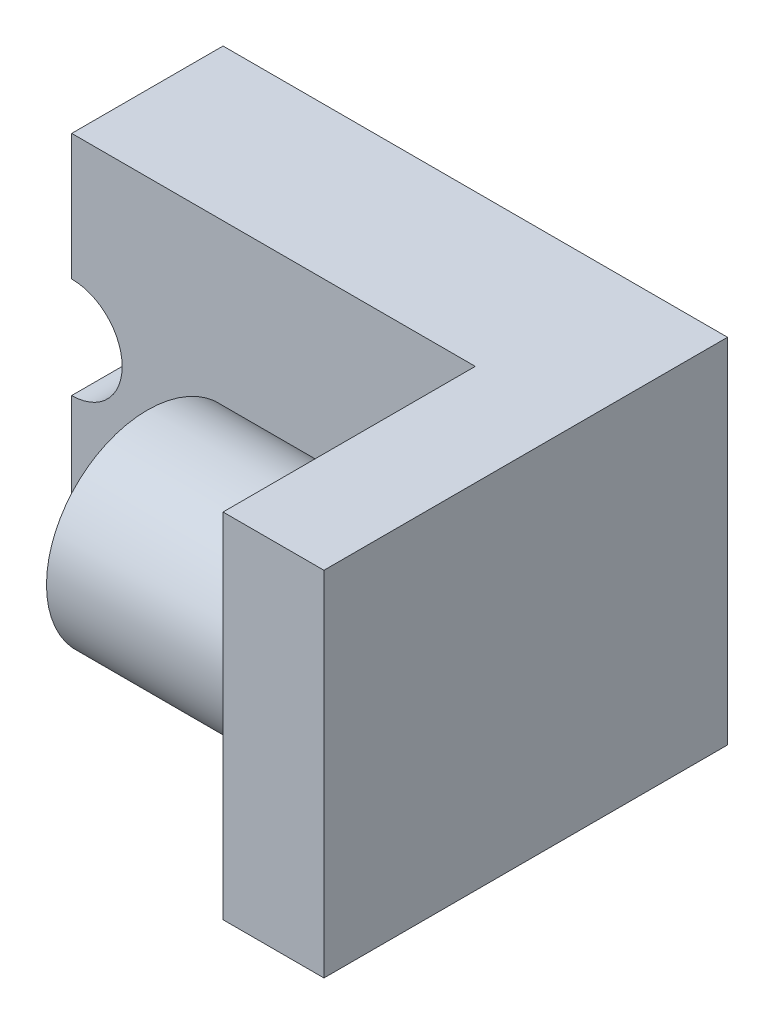
ISO-10303-21;
HEADER;
FILE_DESCRIPTION(('STEP AP214'),'2;1');
FILE_NAME('part.step','',(''),(''),'','','');
FILE_SCHEMA(('AUTOMOTIVE_DESIGN { 1 0 10303 214 1 1 1 1 }'));
ENDSEC;
DATA;
#1=APPLICATION_CONTEXT('core data for automotive mechanical design processes');
#2=APPLICATION_PROTOCOL_DEFINITION('international standard','automotive_design',2000,#1);
#3=PRODUCT_CONTEXT('',#1,'mechanical');
#4=PRODUCT('Part','Part','',(#3));
#5=PRODUCT_RELATED_PRODUCT_CATEGORY('part','',(#4));
#6=PRODUCT_DEFINITION_FORMATION('','',#4);
#7=PRODUCT_DEFINITION_CONTEXT('part definition',#1,'design');
#8=PRODUCT_DEFINITION('design','',#6,#7);
#9=PRODUCT_DEFINITION_SHAPE('','',#8);
#10=(LENGTH_UNIT() NAMED_UNIT(*) SI_UNIT(.MILLI.,.METRE.));
#11=(NAMED_UNIT(*) PLANE_ANGLE_UNIT() SI_UNIT($,.RADIAN.));
#12=(NAMED_UNIT(*) SI_UNIT($,.STERADIAN.) SOLID_ANGLE_UNIT());
#13=UNCERTAINTY_MEASURE_WITH_UNIT(LENGTH_MEASURE(1.E-05),#10,'distance_accuracy_value','');
#14=(GEOMETRIC_REPRESENTATION_CONTEXT(3) GLOBAL_UNCERTAINTY_ASSIGNED_CONTEXT((#13)) GLOBAL_UNIT_ASSIGNED_CONTEXT((#10,
#11,#12)) REPRESENTATION_CONTEXT('',''));
#15=CARTESIAN_POINT('',(0.,0.,0.));
#16=DIRECTION('',(0.,0.,1.));
#17=DIRECTION('',(1.,0.,0.));
#18=AXIS2_PLACEMENT_3D('',#15,#16,#17);
#19=CARTESIAN_POINT('',(0.,0.,30.));
#20=DIRECTION('',(0.,0.,1.));
#21=DIRECTION('',(1.,0.,0.));
#22=AXIS2_PLACEMENT_3D('',#19,#20,#21);
#23=PLANE('',#22);
#24=DIRECTION('',(1.,0.,0.));
#25=VECTOR('',#24,1.);
#26=CARTESIAN_POINT('',(0.,0.,30.));
#27=LINE('',#26,#25);
#28=CARTESIAN_POINT('',(0.,0.,30.));
#29=VERTEX_POINT('',#28);
#30=CARTESIAN_POINT('',(80.,0.,30.));
#31=VERTEX_POINT('',#30);
#32=EDGE_CURVE('E151',#29,#31,#27,.T.);
#33=ORIENTED_EDGE('',*,*,#32,.T.);
#34=DIRECTION('',(0.,1.,0.));
#35=VECTOR('',#34,1.);
#36=CARTESIAN_POINT('',(80.,0.,30.));
#37=LINE('',#36,#35);
#38=CARTESIAN_POINT('',(80.,70.,30.));
#39=VERTEX_POINT('',#38);
#40=EDGE_CURVE('E133',#31,#39,#37,.T.);
#41=ORIENTED_EDGE('',*,*,#40,.T.);
#42=DIRECTION('',(-1.,0.,0.));
#43=VECTOR('',#42,1.);
#44=CARTESIAN_POINT('',(100.,70.,30.));
#45=LINE('',#44,#43);
#46=CARTESIAN_POINT('',(0.,70.,30.));
#47=VERTEX_POINT('',#46);
#48=EDGE_CURVE('E128',#39,#47,#45,.T.);
#49=ORIENTED_EDGE('',*,*,#48,.T.);
#50=DIRECTION('',(0.,-1.,0.));
#51=VECTOR('',#50,1.);
#52=CARTESIAN_POINT('',(0.,70.,30.));
#53=LINE('',#52,#51);
#54=CARTESIAN_POINT('',(0.,45.,30.));
#55=VERTEX_POINT('',#54);
#56=EDGE_CURVE('E146',#47,#55,#53,.T.);
#57=ORIENTED_EDGE('',*,*,#56,.T.);
#58=CARTESIAN_POINT('',(0.,35.,30.));
#59=DIRECTION('',(0.,0.,1.));
#60=DIRECTION('',(1.,0.,0.));
#61=AXIS2_PLACEMENT_3D('',#58,#59,#60);
#62=CIRCLE('',#61,10.);
#63=CARTESIAN_POINT('',(0.,25.,30.));
#64=VERTEX_POINT('',#63);
#65=EDGE_CURVE('E136',#64,#55,#62,.T.);
#66=ORIENTED_EDGE('',*,*,#65,.F.);
#67=EDGE_CURVE('E155',#64,#29,#53,.T.);
#68=ORIENTED_EDGE('',*,*,#67,.T.);
#69=EDGE_LOOP('',(#33,#41,#49,#57,#66,#68));
#70=FACE_BOUND('',#69,.T.);
#71=ADVANCED_FACE('F44',(#70),#23,.T.);
#72=CARTESIAN_POINT('',(0.,70.,30.));
#73=DIRECTION('',(1.,0.,0.));
#74=DIRECTION('',(0.,0.,-1.));
#75=AXIS2_PLACEMENT_3D('',#72,#73,#74);
#76=PLANE('',#75);
#77=DIRECTION('',(0.,-1.,0.));
#78=VECTOR('',#77,1.);
#79=CARTESIAN_POINT('',(0.,70.,0.));
#80=LINE('',#79,#78);
#81=CARTESIAN_POINT('',(0.,70.,0.));
#82=VERTEX_POINT('',#81);
#83=CARTESIAN_POINT('',(0.,45.,0.));
#84=VERTEX_POINT('',#83);
#85=EDGE_CURVE('E160',#82,#84,#80,.T.);
#86=ORIENTED_EDGE('',*,*,#85,.T.);
#87=DIRECTION('',(0.,0.,1.));
#88=VECTOR('',#87,1.);
#89=CARTESIAN_POINT('',(0.,45.,0.));
#90=LINE('',#89,#88);
#91=EDGE_CURVE('E69',#84,#55,#90,.T.);
#92=ORIENTED_EDGE('',*,*,#91,.T.);
#93=ORIENTED_EDGE('',*,*,#56,.F.);
#94=DIRECTION('',(0.,0.,-1.));
#95=VECTOR('',#94,1.);
#96=CARTESIAN_POINT('',(0.,70.,30.));
#97=LINE('',#96,#95);
#98=EDGE_CURVE('E156',#47,#82,#97,.T.);
#99=ORIENTED_EDGE('',*,*,#98,.T.);
#100=EDGE_LOOP('',(#86,#92,#93,#99));
#101=FACE_BOUND('',#100,.T.);
#102=ADVANCED_FACE('F192',(#101),#76,.F.);
#103=ORIENTED_EDGE('',*,*,#67,.F.);
#104=DIRECTION('',(0.,0.,1.));
#105=VECTOR('',#104,1.);
#106=CARTESIAN_POINT('',(0.,25.,0.));
#107=LINE('',#106,#105);
#108=CARTESIAN_POINT('',(0.,25.,0.));
#109=VERTEX_POINT('',#108);
#110=EDGE_CURVE('E145',#109,#64,#107,.T.);
#111=ORIENTED_EDGE('',*,*,#110,.F.);
#112=CARTESIAN_POINT('',(0.,0.,0.));
#113=VERTEX_POINT('',#112);
#114=EDGE_CURVE('E148',#109,#113,#80,.T.);
#115=ORIENTED_EDGE('',*,*,#114,.T.);
#116=DIRECTION('',(0.,0.,-1.));
#117=VECTOR('',#116,1.);
#118=CARTESIAN_POINT('',(0.,0.,30.));
#119=LINE('',#118,#117);
#120=EDGE_CURVE('E52',#29,#113,#119,.T.);
#121=ORIENTED_EDGE('',*,*,#120,.F.);
#122=EDGE_LOOP('',(#103,#111,#115,#121));
#123=FACE_BOUND('',#122,.T.);
#124=ADVANCED_FACE('F50',(#123),#76,.F.);
#125=CARTESIAN_POINT('',(0.,0.,30.));
#126=DIRECTION('',(0.,1.,0.));
#127=DIRECTION('',(0.,0.,1.));
#128=AXIS2_PLACEMENT_3D('',#125,#126,#127);
#129=PLANE('',#128);
#130=DIRECTION('',(1.,0.,0.));
#131=VECTOR('',#130,1.);
#132=CARTESIAN_POINT('',(0.,0.,0.));
#133=LINE('',#132,#131);
#134=CARTESIAN_POINT('',(100.,0.,0.));
#135=VERTEX_POINT('',#134);
#136=EDGE_CURVE('E159',#113,#135,#133,.T.);
#137=ORIENTED_EDGE('',*,*,#136,.T.);
#138=DIRECTION('',(0.,0.,-1.));
#139=VECTOR('',#138,1.);
#140=CARTESIAN_POINT('',(100.,0.,30.));
#141=LINE('',#140,#139);
#142=CARTESIAN_POINT('',(100.,0.,80.));
#143=VERTEX_POINT('',#142);
#144=EDGE_CURVE('E168',#143,#135,#141,.T.);
#145=ORIENTED_EDGE('',*,*,#144,.F.);
#146=DIRECTION('',(1.,0.,0.));
#147=VECTOR('',#146,1.);
#148=CARTESIAN_POINT('',(80.,0.,80.));
#149=LINE('',#148,#147);
#150=CARTESIAN_POINT('',(80.,0.,80.));
#151=VERTEX_POINT('',#150);
#152=EDGE_CURVE('E122',#151,#143,#149,.T.);
#153=ORIENTED_EDGE('',*,*,#152,.F.);
#154=DIRECTION('',(0.,0.,-1.));
#155=VECTOR('',#154,1.);
#156=CARTESIAN_POINT('',(80.,0.,80.));
#157=LINE('',#156,#155);
#158=EDGE_CURVE('E125',#151,#31,#157,.T.);
#159=ORIENTED_EDGE('',*,*,#158,.T.);
#160=ORIENTED_EDGE('',*,*,#32,.F.);
#161=ORIENTED_EDGE('',*,*,#120,.T.);
#162=EDGE_LOOP('',(#137,#145,#153,#159,#160,#161));
#163=FACE_BOUND('',#162,.T.);
#164=ADVANCED_FACE('F177',(#163),#129,.F.);
#165=CARTESIAN_POINT('',(100.,0.,30.));
#166=DIRECTION('',(-1.,0.,0.));
#167=DIRECTION('',(0.,0.,1.));
#168=AXIS2_PLACEMENT_3D('',#165,#166,#167);
#169=PLANE('',#168);
#170=DIRECTION('',(0.,1.,0.));
#171=VECTOR('',#170,1.);
#172=CARTESIAN_POINT('',(100.,0.,0.));
#173=LINE('',#172,#171);
#174=CARTESIAN_POINT('',(100.,70.,0.));
#175=VERTEX_POINT('',#174);
#176=EDGE_CURVE('E165',#135,#175,#173,.T.);
#177=ORIENTED_EDGE('',*,*,#176,.T.);
#178=DIRECTION('',(0.,0.,-1.));
#179=VECTOR('',#178,1.);
#180=CARTESIAN_POINT('',(100.,70.,30.));
#181=LINE('',#180,#179);
#182=CARTESIAN_POINT('',(100.,70.,80.));
#183=VERTEX_POINT('',#182);
#184=EDGE_CURVE('E169',#183,#175,#181,.T.);
#185=ORIENTED_EDGE('',*,*,#184,.F.);
#186=DIRECTION('',(0.,-1.,0.));
#187=VECTOR('',#186,1.);
#188=CARTESIAN_POINT('',(100.,70.,80.));
#189=LINE('',#188,#187);
#190=EDGE_CURVE('E116',#183,#143,#189,.T.);
#191=ORIENTED_EDGE('',*,*,#190,.T.);
#192=ORIENTED_EDGE('',*,*,#144,.T.);
#193=EDGE_LOOP('',(#177,#185,#191,#192));
#194=FACE_BOUND('',#193,.T.);
#195=ADVANCED_FACE('F186',(#194),#169,.F.);
#196=CARTESIAN_POINT('',(100.,70.,30.));
#197=DIRECTION('',(0.,-1.,0.));
#198=DIRECTION('',(0.,0.,-1.));
#199=AXIS2_PLACEMENT_3D('',#196,#197,#198);
#200=PLANE('',#199);
#201=DIRECTION('',(-1.,0.,0.));
#202=VECTOR('',#201,1.);
#203=CARTESIAN_POINT('',(100.,70.,0.));
#204=LINE('',#203,#202);
#205=EDGE_CURVE('E163',#175,#82,#204,.T.);
#206=ORIENTED_EDGE('',*,*,#205,.T.);
#207=ORIENTED_EDGE('',*,*,#98,.F.);
#208=ORIENTED_EDGE('',*,*,#48,.F.);
#209=DIRECTION('',(0.,0.,1.));
#210=VECTOR('',#209,1.);
#211=CARTESIAN_POINT('',(80.,70.,30.));
#212=LINE('',#211,#210);
#213=CARTESIAN_POINT('',(80.,70.,80.));
#214=VERTEX_POINT('',#213);
#215=EDGE_CURVE('E58',#39,#214,#212,.T.);
#216=ORIENTED_EDGE('',*,*,#215,.T.);
#217=DIRECTION('',(1.,0.,0.));
#218=VECTOR('',#217,1.);
#219=CARTESIAN_POINT('',(80.,70.,80.));
#220=LINE('',#219,#218);
#221=EDGE_CURVE('E115',#214,#183,#220,.T.);
#222=ORIENTED_EDGE('',*,*,#221,.T.);
#223=ORIENTED_EDGE('',*,*,#184,.T.);
#224=EDGE_LOOP('',(#206,#207,#208,#216,#222,#223));
#225=FACE_BOUND('',#224,.T.);
#226=ADVANCED_FACE('F126',(#225),#200,.F.);
#227=CARTESIAN_POINT('',(0.,0.,0.));
#228=DIRECTION('',(0.,0.,1.));
#229=DIRECTION('',(1.,0.,0.));
#230=AXIS2_PLACEMENT_3D('',#227,#228,#229);
#231=PLANE('',#230);
#232=ORIENTED_EDGE('',*,*,#114,.F.);
#233=CARTESIAN_POINT('',(0.,35.,0.));
#234=DIRECTION('',(0.,0.,1.));
#235=DIRECTION('',(1.,0.,0.));
#236=AXIS2_PLACEMENT_3D('',#233,#234,#235);
#237=CIRCLE('',#236,10.);
#238=EDGE_CURVE('E143',#109,#84,#237,.T.);
#239=ORIENTED_EDGE('',*,*,#238,.T.);
#240=ORIENTED_EDGE('',*,*,#85,.F.);
#241=ORIENTED_EDGE('',*,*,#205,.F.);
#242=ORIENTED_EDGE('',*,*,#176,.F.);
#243=ORIENTED_EDGE('',*,*,#136,.F.);
#244=EDGE_LOOP('',(#232,#239,#240,#241,#242,#243));
#245=FACE_BOUND('',#244,.T.);
#246=ADVANCED_FACE('F184',(#245),#231,.F.);
#247=CARTESIAN_POINT('',(0.,35.,0.));
#248=DIRECTION('',(0.,0.,1.));
#249=DIRECTION('',(1.,0.,0.));
#250=AXIS2_PLACEMENT_3D('',#247,#248,#249);
#251=CYLINDRICAL_SURFACE('',#250,10.);
#252=ORIENTED_EDGE('',*,*,#65,.T.);
#253=ORIENTED_EDGE('',*,*,#91,.F.);
#254=ORIENTED_EDGE('',*,*,#238,.F.);
#255=ORIENTED_EDGE('',*,*,#110,.T.);
#256=EDGE_LOOP('',(#252,#253,#254,#255));
#257=FACE_BOUND('',#256,.T.);
#258=ADVANCED_FACE('F195',(#257),#251,.F.);
#259=CARTESIAN_POINT('',(80.,70.,80.));
#260=DIRECTION('',(0.,0.,1.));
#261=DIRECTION('',(1.,0.,0.));
#262=AXIS2_PLACEMENT_3D('',#259,#260,#261);
#263=PLANE('',#262);
#264=ORIENTED_EDGE('',*,*,#190,.F.);
#265=ORIENTED_EDGE('',*,*,#221,.F.);
#266=DIRECTION('',(0.,-1.,0.));
#267=VECTOR('',#266,1.);
#268=CARTESIAN_POINT('',(80.,70.,80.));
#269=LINE('',#268,#267);
#270=EDGE_CURVE('E113',#214,#151,#269,.T.);
#271=ORIENTED_EDGE('',*,*,#270,.T.);
#272=ORIENTED_EDGE('',*,*,#152,.T.);
#273=EDGE_LOOP('',(#264,#265,#271,#272));
#274=FACE_BOUND('',#273,.T.);
#275=ADVANCED_FACE('F114',(#274),#263,.T.);
#276=CARTESIAN_POINT('',(80.,0.,0.));
#277=DIRECTION('',(1.,0.,0.));
#278=DIRECTION('',(0.,0.,-1.));
#279=AXIS2_PLACEMENT_3D('',#276,#277,#278);
#280=PLANE('',#279);
#281=CARTESIAN_POINT('',(80.,35.,55.));
#282=DIRECTION('',(1.,0.,0.));
#283=DIRECTION('',(0.,0.,-1.));
#284=AXIS2_PLACEMENT_3D('',#281,#282,#283);
#285=CIRCLE('',#284,20.);
#286=CARTESIAN_POINT('',(80.,35.,35.));
#287=VERTEX_POINT('',#286);
#288=EDGE_CURVE('E11',#287,#287,#285,.F.);
#289=ORIENTED_EDGE('',*,*,#288,.F.);
#290=EDGE_LOOP('',(#289));
#291=FACE_BOUND('',#290,.T.);
#292=ORIENTED_EDGE('',*,*,#40,.F.);
#293=ORIENTED_EDGE('',*,*,#158,.F.);
#294=ORIENTED_EDGE('',*,*,#270,.F.);
#295=ORIENTED_EDGE('',*,*,#215,.F.);
#296=EDGE_LOOP('',(#292,#293,#294,#295));
#297=FACE_BOUND('',#296,.T.);
#298=ADVANCED_FACE('F121',(#291,#297),#280,.F.);
#299=CARTESIAN_POINT('',(40.,35.,55.));
#300=DIRECTION('',(-1.,0.,0.));
#301=DIRECTION('',(0.,0.,1.));
#302=AXIS2_PLACEMENT_3D('',#299,#300,#301);
#303=PLANE('',#302);
#304=CARTESIAN_POINT('',(40.,35.,55.));
#305=DIRECTION('',(-1.,0.,0.));
#306=DIRECTION('',(0.,0.,1.));
#307=AXIS2_PLACEMENT_3D('',#304,#305,#306);
#308=CIRCLE('',#307,20.);
#309=CARTESIAN_POINT('',(40.,35.,75.));
#310=VERTEX_POINT('',#309);
#311=EDGE_CURVE('E139',#310,#310,#308,.T.);
#312=ORIENTED_EDGE('',*,*,#311,.T.);
#313=EDGE_LOOP('',(#312));
#314=FACE_BOUND('',#313,.T.);
#315=CARTESIAN_POINT('',(40.,35.,55.));
#316=DIRECTION('',(-1.,0.,0.));
#317=DIRECTION('',(0.,0.,1.));
#318=AXIS2_PLACEMENT_3D('',#315,#316,#317);
#319=CIRCLE('',#318,10.);
#320=CARTESIAN_POINT('',(40.,35.,65.));
#321=VERTEX_POINT('',#320);
#322=EDGE_CURVE('E374',#321,#321,#319,.T.);
#323=ORIENTED_EDGE('',*,*,#322,.F.);
#324=EDGE_LOOP('',(#323));
#325=FACE_BOUND('',#324,.T.);
#326=ADVANCED_FACE('F260',(#314,#325),#303,.T.);
#327=CARTESIAN_POINT('',(40.,35.,55.));
#328=DIRECTION('',(1.,0.,0.));
#329=DIRECTION('',(0.,0.,-1.));
#330=AXIS2_PLACEMENT_3D('',#327,#328,#329);
#331=CYLINDRICAL_SURFACE('',#330,20.);
#332=ORIENTED_EDGE('',*,*,#311,.F.);
#333=EDGE_LOOP('',(#332));
#334=FACE_BOUND('',#333,.T.);
#335=ORIENTED_EDGE('',*,*,#288,.T.);
#336=EDGE_LOOP('',(#335));
#337=FACE_BOUND('',#336,.T.);
#338=ADVANCED_FACE('F261',(#334,#337),#331,.T.);
#339=CARTESIAN_POINT('',(40.,35.,55.));
#340=DIRECTION('',(1.,0.,0.));
#341=DIRECTION('',(0.,0.,-1.));
#342=AXIS2_PLACEMENT_3D('',#339,#340,#341);
#343=CYLINDRICAL_SURFACE('',#342,10.);
#344=ORIENTED_EDGE('',*,*,#322,.T.);
#345=EDGE_LOOP('',(#344));
#346=FACE_BOUND('',#345,.T.);
#347=CARTESIAN_POINT('',(80.,35.,55.));
#348=DIRECTION('',(-1.,0.,0.));
#349=DIRECTION('',(0.,0.,1.));
#350=AXIS2_PLACEMENT_3D('',#347,#348,#349);
#351=CIRCLE('',#350,10.);
#352=CARTESIAN_POINT('',(80.,35.,65.));
#353=VERTEX_POINT('',#352);
#354=EDGE_CURVE('E373',#353,#353,#351,.T.);
#355=ORIENTED_EDGE('',*,*,#354,.F.);
#356=EDGE_LOOP('',(#355));
#357=FACE_BOUND('',#356,.T.);
#358=ADVANCED_FACE('F275',(#346,#357),#343,.F.);
#359=ORIENTED_EDGE('',*,*,#354,.T.);
#360=EDGE_LOOP('',(#359));
#361=FACE_BOUND('',#360,.T.);
#362=ADVANCED_FACE('F283',(#361),#280,.F.);
#363=CLOSED_SHELL('',(#71,#102,#124,#164,#195,#226,#246,#258,#275,#298,#326,#338,#358,#362));
#364=MANIFOLD_SOLID_BREP('B2',#363);
#365=ADVANCED_BREP_SHAPE_REPRESENTATION('',(#18,#364),#14);
#366=SHAPE_DEFINITION_REPRESENTATION(#9,#365);
ENDSEC;
END-ISO-10303-21;
